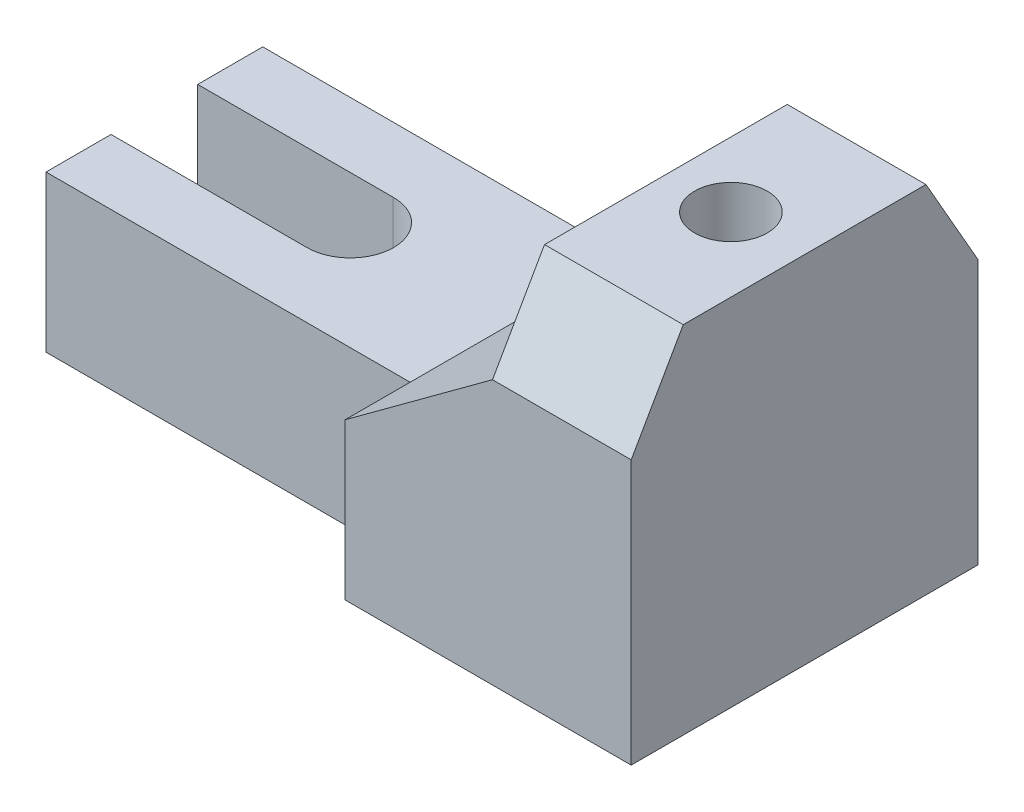
ISO-10303-21;
HEADER;
FILE_DESCRIPTION(('STEP AP214'),'2;1');
FILE_NAME('part.step','',(''),(''),'','','');
FILE_SCHEMA(('AUTOMOTIVE_DESIGN { 1 0 10303 214 1 1 1 1 }'));
ENDSEC;
DATA;
#1=APPLICATION_CONTEXT('core data for automotive mechanical design processes');
#2=APPLICATION_PROTOCOL_DEFINITION('international standard','automotive_design',2000,#1);
#3=PRODUCT_CONTEXT('',#1,'mechanical');
#4=PRODUCT('Part','Part','',(#3));
#5=PRODUCT_RELATED_PRODUCT_CATEGORY('part','',(#4));
#6=PRODUCT_DEFINITION_FORMATION('','',#4);
#7=PRODUCT_DEFINITION_CONTEXT('part definition',#1,'design');
#8=PRODUCT_DEFINITION('design','',#6,#7);
#9=PRODUCT_DEFINITION_SHAPE('','',#8);
#10=(LENGTH_UNIT() NAMED_UNIT(*) SI_UNIT(.MILLI.,.METRE.));
#11=(NAMED_UNIT(*) PLANE_ANGLE_UNIT() SI_UNIT($,.RADIAN.));
#12=(NAMED_UNIT(*) SI_UNIT($,.STERADIAN.) SOLID_ANGLE_UNIT());
#13=UNCERTAINTY_MEASURE_WITH_UNIT(LENGTH_MEASURE(1.E-05),#10,'distance_accuracy_value','');
#14=(GEOMETRIC_REPRESENTATION_CONTEXT(3) GLOBAL_UNCERTAINTY_ASSIGNED_CONTEXT((#13)) GLOBAL_UNIT_ASSIGNED_CONTEXT((#10,
#11,#12)) REPRESENTATION_CONTEXT('',''));
#15=CARTESIAN_POINT('',(0.,0.,0.));
#16=DIRECTION('',(0.,0.,1.));
#17=DIRECTION('',(1.,0.,0.));
#18=AXIS2_PLACEMENT_3D('',#15,#16,#17);
#19=CARTESIAN_POINT('',(-39.,0.,0.));
#20=DIRECTION('',(-1.,0.,0.));
#21=DIRECTION('',(0.,0.,1.));
#22=AXIS2_PLACEMENT_3D('',#19,#20,#21);
#23=PLANE('',#22);
#24=DIRECTION('',(0.,1.,0.));
#25=VECTOR('',#24,1.);
#26=CARTESIAN_POINT('',(-39.,0.,9.99809322082355));
#27=LINE('',#26,#25);
#28=CARTESIAN_POINT('',(-39.,0.,9.99809322082355));
#29=VERTEX_POINT('',#28);
#30=CARTESIAN_POINT('',(-39.,36.,9.99809322082355));
#31=VERTEX_POINT('',#30);
#32=EDGE_CURVE('E11',#29,#31,#27,.T.);
#33=ORIENTED_EDGE('',*,*,#32,.F.);
#34=DIRECTION('',(0.,0.,1.));
#35=VECTOR('',#34,1.);
#36=CARTESIAN_POINT('',(-39.,0.,-10.));
#37=LINE('',#36,#35);
#38=CARTESIAN_POINT('',(-39.,0.,10.));
#39=VERTEX_POINT('',#38);
#40=EDGE_CURVE('E291',#29,#39,#37,.T.);
#41=ORIENTED_EDGE('',*,*,#40,.T.);
#42=DIRECTION('',(0.,1.,0.));
#43=VECTOR('',#42,1.);
#44=CARTESIAN_POINT('',(-39.,36.,9.99999999999999));
#45=LINE('',#44,#43);
#46=CARTESIAN_POINT('',(-39.,36.,9.99999999999999));
#47=VERTEX_POINT('',#46);
#48=EDGE_CURVE('E173',#39,#47,#45,.T.);
#49=ORIENTED_EDGE('',*,*,#48,.T.);
#50=DIRECTION('',(0.,0.,-1.));
#51=VECTOR('',#50,1.);
#52=CARTESIAN_POINT('',(-39.,36.,-10.));
#53=LINE('',#52,#51);
#54=EDGE_CURVE('E170',#47,#31,#53,.T.);
#55=ORIENTED_EDGE('',*,*,#54,.T.);
#56=EDGE_LOOP('',(#33,#41,#49,#55));
#57=FACE_BOUND('',#56,.T.);
#58=ADVANCED_FACE('F39',(#57),#23,.T.);
#59=CARTESIAN_POINT('',(-84.,0.,0.));
#60=DIRECTION('',(-1.,0.,0.));
#61=DIRECTION('',(0.,0.,1.));
#62=AXIS2_PLACEMENT_3D('',#59,#60,#61);
#63=PLANE('',#62);
#64=DIRECTION('',(0.,-1.,0.));
#65=VECTOR('',#64,1.);
#66=CARTESIAN_POINT('',(-84.,36.,-10.));
#67=LINE('',#66,#65);
#68=CARTESIAN_POINT('',(-84.,36.,-10.));
#69=VERTEX_POINT('',#68);
#70=CARTESIAN_POINT('',(-84.,0.,-10.));
#71=VERTEX_POINT('',#70);
#72=EDGE_CURVE('E181',#69,#71,#67,.T.);
#73=ORIENTED_EDGE('',*,*,#72,.F.);
#74=DIRECTION('',(0.,0.,-1.));
#75=VECTOR('',#74,1.);
#76=CARTESIAN_POINT('',(-84.,36.,-25.));
#77=LINE('',#76,#75);
#78=CARTESIAN_POINT('',(-84.,36.,-25.));
#79=VERTEX_POINT('',#78);
#80=EDGE_CURVE('E205',#69,#79,#77,.T.);
#81=ORIENTED_EDGE('',*,*,#80,.T.);
#82=DIRECTION('',(0.,-1.,0.));
#83=VECTOR('',#82,1.);
#84=CARTESIAN_POINT('',(-84.,36.,-25.));
#85=LINE('',#84,#83);
#86=CARTESIAN_POINT('',(-84.,0.,-25.));
#87=VERTEX_POINT('',#86);
#88=EDGE_CURVE('E195',#79,#87,#85,.T.);
#89=ORIENTED_EDGE('',*,*,#88,.T.);
#90=DIRECTION('',(0.,0.,1.));
#91=VECTOR('',#90,1.);
#92=CARTESIAN_POINT('',(-84.,0.,-25.));
#93=LINE('',#92,#91);
#94=EDGE_CURVE('E196',#87,#71,#93,.T.);
#95=ORIENTED_EDGE('',*,*,#94,.T.);
#96=EDGE_LOOP('',(#73,#81,#89,#95));
#97=FACE_BOUND('',#96,.T.);
#98=ADVANCED_FACE('F324',(#97),#63,.T.);
#99=CARTESIAN_POINT('',(0.,0.,40.));
#100=DIRECTION('',(1.,0.,0.));
#101=DIRECTION('',(0.,0.,-1.));
#102=AXIS2_PLACEMENT_3D('',#99,#100,#101);
#103=PLANE('',#102);
#104=DIRECTION('',(0.,-1.,0.));
#105=VECTOR('',#104,1.);
#106=CARTESIAN_POINT('',(0.,36.,-25.));
#107=LINE('',#106,#105);
#108=CARTESIAN_POINT('',(0.,36.,-25.));
#109=VERTEX_POINT('',#108);
#110=CARTESIAN_POINT('',(0.,0.,-25.));
#111=VERTEX_POINT('',#110);
#112=EDGE_CURVE('E189',#109,#111,#107,.T.);
#113=ORIENTED_EDGE('',*,*,#112,.F.);
#114=DIRECTION('',(0.,0.,-1.));
#115=VECTOR('',#114,1.);
#116=CARTESIAN_POINT('',(0.,36.,40.));
#117=LINE('',#116,#115);
#118=CARTESIAN_POINT('',(0.,36.,-40.));
#119=VERTEX_POINT('',#118);
#120=EDGE_CURVE('E278',#109,#119,#117,.T.);
#121=ORIENTED_EDGE('',*,*,#120,.T.);
#122=DIRECTION('',(0.,-1.,0.));
#123=VECTOR('',#122,1.);
#124=CARTESIAN_POINT('',(0.,0.,-40.));
#125=LINE('',#124,#123);
#126=CARTESIAN_POINT('',(0.,0.,-40.));
#127=VERTEX_POINT('',#126);
#128=EDGE_CURVE('E256',#119,#127,#125,.T.);
#129=ORIENTED_EDGE('',*,*,#128,.T.);
#130=DIRECTION('',(0.,0.,-1.));
#131=VECTOR('',#130,1.);
#132=CARTESIAN_POINT('',(0.,0.,40.));
#133=LINE('',#132,#131);
#134=EDGE_CURVE('E266',#111,#127,#133,.T.);
#135=ORIENTED_EDGE('',*,*,#134,.F.);
#136=EDGE_LOOP('',(#113,#121,#129,#135));
#137=FACE_BOUND('',#136,.T.);
#138=ADVANCED_FACE('F327',(#137),#103,.F.);
#139=DIRECTION('',(0.,1.,0.));
#140=VECTOR('',#139,1.);
#141=CARTESIAN_POINT('',(0.,36.,25.));
#142=LINE('',#141,#140);
#143=CARTESIAN_POINT('',(0.,0.,25.));
#144=VERTEX_POINT('',#143);
#145=CARTESIAN_POINT('',(0.,36.,25.));
#146=VERTEX_POINT('',#145);
#147=EDGE_CURVE('E209',#144,#146,#142,.T.);
#148=ORIENTED_EDGE('',*,*,#147,.F.);
#149=CARTESIAN_POINT('',(0.,0.,40.));
#150=VERTEX_POINT('',#149);
#151=EDGE_CURVE('E280',#150,#144,#133,.T.);
#152=ORIENTED_EDGE('',*,*,#151,.F.);
#153=DIRECTION('',(0.,-1.,0.));
#154=VECTOR('',#153,1.);
#155=CARTESIAN_POINT('',(0.,0.,40.));
#156=LINE('',#155,#154);
#157=CARTESIAN_POINT('',(0.,36.,40.));
#158=VERTEX_POINT('',#157);
#159=EDGE_CURVE('E263',#158,#150,#156,.T.);
#160=ORIENTED_EDGE('',*,*,#159,.F.);
#161=EDGE_CURVE('E284',#158,#146,#117,.T.);
#162=ORIENTED_EDGE('',*,*,#161,.T.);
#163=EDGE_LOOP('',(#148,#152,#160,#162));
#164=FACE_BOUND('',#163,.T.);
#165=ADVANCED_FACE('F405',(#164),#103,.F.);
#166=CARTESIAN_POINT('',(66.,0.,40.));
#167=DIRECTION('',(0.,1.,0.));
#168=DIRECTION('',(0.,0.,1.));
#169=AXIS2_PLACEMENT_3D('',#166,#167,#168);
#170=PLANE('',#169);
#171=CARTESIAN_POINT('',(49.,0.,0.));
#172=DIRECTION('',(0.,1.,0.));
#173=DIRECTION('',(0.,0.,1.));
#174=AXIS2_PLACEMENT_3D('',#171,#172,#173);
#175=CIRCLE('',#174,8.38186830152186);
#176=CARTESIAN_POINT('',(49.,0.,-8.38186830152186));
#177=VERTEX_POINT('',#176);
#178=EDGE_CURVE('E167',#177,#177,#175,.T.);
#179=ORIENTED_EDGE('',*,*,#178,.T.);
#180=EDGE_LOOP('',(#179));
#181=FACE_BOUND('',#180,.T.);
#182=ORIENTED_EDGE('',*,*,#40,.F.);
#183=CARTESIAN_POINT('',(-38.8047259676192,0.,0.));
#184=DIRECTION('',(0.,1.,0.));
#185=DIRECTION('',(0.,0.,1.));
#186=AXIS2_PLACEMENT_3D('',#183,#184,#185);
#187=CIRCLE('',#186,10.);
#188=CARTESIAN_POINT('',(-39.,0.,-9.99809322082355));
#189=VERTEX_POINT('',#188);
#190=EDGE_CURVE('E157',#29,#189,#187,.T.);
#191=ORIENTED_EDGE('',*,*,#190,.T.);
#192=CARTESIAN_POINT('',(-39.,0.,-10.));
#193=VERTEX_POINT('',#192);
#194=EDGE_CURVE('E292',#193,#189,#37,.T.);
#195=ORIENTED_EDGE('',*,*,#194,.F.);
#196=DIRECTION('',(-1.,0.,0.));
#197=VECTOR('',#196,1.);
#198=CARTESIAN_POINT('',(-39.,0.,-10.));
#199=LINE('',#198,#197);
#200=EDGE_CURVE('E172',#193,#71,#199,.T.);
#201=ORIENTED_EDGE('',*,*,#200,.T.);
#202=ORIENTED_EDGE('',*,*,#94,.F.);
#203=DIRECTION('',(1.,0.,0.));
#204=VECTOR('',#203,1.);
#205=CARTESIAN_POINT('',(-84.,0.,-25.));
#206=LINE('',#205,#204);
#207=EDGE_CURVE('E225',#87,#111,#206,.T.);
#208=ORIENTED_EDGE('',*,*,#207,.T.);
#209=ORIENTED_EDGE('',*,*,#134,.T.);
#210=DIRECTION('',(1.,0.,0.));
#211=VECTOR('',#210,1.);
#212=CARTESIAN_POINT('',(66.,0.,-40.));
#213=LINE('',#212,#211);
#214=CARTESIAN_POINT('',(66.,0.,-40.));
#215=VERTEX_POINT('',#214);
#216=EDGE_CURVE('E251',#127,#215,#213,.T.);
#217=ORIENTED_EDGE('',*,*,#216,.T.);
#218=DIRECTION('',(0.,0.,-1.));
#219=VECTOR('',#218,1.);
#220=CARTESIAN_POINT('',(66.,0.,40.));
#221=LINE('',#220,#219);
#222=CARTESIAN_POINT('',(66.,0.,40.));
#223=VERTEX_POINT('',#222);
#224=EDGE_CURVE('E286',#223,#215,#221,.T.);
#225=ORIENTED_EDGE('',*,*,#224,.F.);
#226=DIRECTION('',(1.,0.,0.));
#227=VECTOR('',#226,1.);
#228=CARTESIAN_POINT('',(66.,0.,40.));
#229=LINE('',#228,#227);
#230=EDGE_CURVE('E253',#150,#223,#229,.T.);
#231=ORIENTED_EDGE('',*,*,#230,.F.);
#232=ORIENTED_EDGE('',*,*,#151,.T.);
#233=DIRECTION('',(1.,0.,0.));
#234=VECTOR('',#233,1.);
#235=CARTESIAN_POINT('',(-84.,0.,25.));
#236=LINE('',#235,#234);
#237=CARTESIAN_POINT('',(-84.,0.,25.));
#238=VERTEX_POINT('',#237);
#239=EDGE_CURVE('E218',#238,#144,#236,.T.);
#240=ORIENTED_EDGE('',*,*,#239,.F.);
#241=CARTESIAN_POINT('',(-84.,0.,10.));
#242=VERTEX_POINT('',#241);
#243=EDGE_CURVE('E193',#242,#238,#93,.T.);
#244=ORIENTED_EDGE('',*,*,#243,.F.);
#245=DIRECTION('',(-1.,0.,0.));
#246=VECTOR('',#245,1.);
#247=CARTESIAN_POINT('',(-39.,0.,10.));
#248=LINE('',#247,#246);
#249=EDGE_CURVE('E62',#39,#242,#248,.T.);
#250=ORIENTED_EDGE('',*,*,#249,.F.);
#251=EDGE_LOOP('',(#182,#191,#195,#201,#202,#208,#209,#217,#225,#231,#232,#240,#244,#250));
#252=FACE_BOUND('',#251,.T.);
#253=ADVANCED_FACE('F41',(#181,#252),#170,.F.);
#254=CARTESIAN_POINT('',(66.,61.,40.));
#255=DIRECTION('',(-1.,0.,0.));
#256=DIRECTION('',(0.,-1.,0.));
#257=AXIS2_PLACEMENT_3D('',#254,#255,#256);
#258=PLANE('',#257);
#259=DIRECTION('',(0.,0.,-1.));
#260=VECTOR('',#259,1.);
#261=CARTESIAN_POINT('',(66.,82.,-40.));
#262=LINE('',#261,#260);
#263=CARTESIAN_POINT('',(66.,82.,28.));
#264=VERTEX_POINT('',#263);
#265=CARTESIAN_POINT('',(66.,82.,-28.));
#266=VERTEX_POINT('',#265);
#267=EDGE_CURVE('E252',#264,#266,#262,.T.);
#268=ORIENTED_EDGE('',*,*,#267,.F.);
#269=DIRECTION('',(0.,0.868243142124459,-0.496138938356834));
#270=VECTOR('',#269,1.);
#271=CARTESIAN_POINT('',(66.,61.,40.));
#272=LINE('',#271,#270);
#273=CARTESIAN_POINT('',(66.,61.,40.));
#274=VERTEX_POINT('',#273);
#275=EDGE_CURVE('E229',#274,#264,#272,.T.);
#276=ORIENTED_EDGE('',*,*,#275,.F.);
#277=DIRECTION('',(0.,1.,0.));
#278=VECTOR('',#277,1.);
#279=CARTESIAN_POINT('',(66.,61.,40.));
#280=LINE('',#279,#278);
#281=EDGE_CURVE('E259',#223,#274,#280,.T.);
#282=ORIENTED_EDGE('',*,*,#281,.F.);
#283=ORIENTED_EDGE('',*,*,#224,.T.);
#284=DIRECTION('',(0.,1.,0.));
#285=VECTOR('',#284,1.);
#286=CARTESIAN_POINT('',(66.,61.,-40.));
#287=LINE('',#286,#285);
#288=CARTESIAN_POINT('',(66.,61.,-40.));
#289=VERTEX_POINT('',#288);
#290=EDGE_CURVE('E268',#215,#289,#287,.T.);
#291=ORIENTED_EDGE('',*,*,#290,.T.);
#292=DIRECTION('',(0.,-0.868243142124459,-0.496138938356834));
#293=VECTOR('',#292,1.);
#294=CARTESIAN_POINT('',(66.,61.,-40.));
#295=LINE('',#294,#293);
#296=EDGE_CURVE('E235',#266,#289,#295,.T.);
#297=ORIENTED_EDGE('',*,*,#296,.F.);
#298=EDGE_LOOP('',(#268,#276,#282,#283,#291,#297));
#299=FACE_BOUND('',#298,.T.);
#300=ADVANCED_FACE('F373',(#299),#258,.F.);
#301=CARTESIAN_POINT('',(0.,36.,40.));
#302=DIRECTION('',(0.592390450477518,-0.805651012649425,0.));
#303=DIRECTION('',(0.805651012649425,0.592390450477518,0.));
#304=AXIS2_PLACEMENT_3D('',#301,#302,#303);
#305=PLANE('',#304);
#306=DIRECTION('',(-0.805651012649425,-0.592390450477518,0.));
#307=VECTOR('',#306,1.);
#308=CARTESIAN_POINT('',(0.,36.,-40.));
#309=LINE('',#308,#307);
#310=CARTESIAN_POINT('',(34.,61.,-40.));
#311=VERTEX_POINT('',#310);
#312=EDGE_CURVE('E275',#311,#119,#309,.T.);
#313=ORIENTED_EDGE('',*,*,#312,.T.);
#314=ORIENTED_EDGE('',*,*,#120,.F.);
#315=DIRECTION('',(0.,0.,-1.));
#316=VECTOR('',#315,1.);
#317=CARTESIAN_POINT('',(0.,36.,-25.));
#318=LINE('',#317,#316);
#319=EDGE_CURVE('E199',#146,#109,#318,.T.);
#320=ORIENTED_EDGE('',*,*,#319,.F.);
#321=ORIENTED_EDGE('',*,*,#161,.F.);
#322=DIRECTION('',(-0.805651012649425,-0.592390450477518,0.));
#323=VECTOR('',#322,1.);
#324=CARTESIAN_POINT('',(0.,36.,40.));
#325=LINE('',#324,#323);
#326=CARTESIAN_POINT('',(34.,61.,40.));
#327=VERTEX_POINT('',#326);
#328=EDGE_CURVE('E261',#327,#158,#325,.T.);
#329=ORIENTED_EDGE('',*,*,#328,.F.);
#330=DIRECTION('',(0.,0.,-1.));
#331=VECTOR('',#330,1.);
#332=CARTESIAN_POINT('',(34.,61.,40.));
#333=LINE('',#332,#331);
#334=EDGE_CURVE('E285',#327,#311,#333,.T.);
#335=ORIENTED_EDGE('',*,*,#334,.T.);
#336=EDGE_LOOP('',(#313,#314,#320,#321,#329,#335));
#337=FACE_BOUND('',#336,.T.);
#338=ADVANCED_FACE('F384',(#337),#305,.F.);
#339=CARTESIAN_POINT('',(0.,0.,40.));
#340=DIRECTION('',(0.,0.,-1.));
#341=DIRECTION('',(-1.,0.,0.));
#342=AXIS2_PLACEMENT_3D('',#339,#340,#341);
#343=PLANE('',#342);
#344=ORIENTED_EDGE('',*,*,#281,.T.);
#345=DIRECTION('',(1.,0.,0.));
#346=VECTOR('',#345,1.);
#347=CARTESIAN_POINT('',(34.,61.,40.));
#348=LINE('',#347,#346);
#349=EDGE_CURVE('E230',#327,#274,#348,.T.);
#350=ORIENTED_EDGE('',*,*,#349,.F.);
#351=ORIENTED_EDGE('',*,*,#328,.T.);
#352=ORIENTED_EDGE('',*,*,#159,.T.);
#353=ORIENTED_EDGE('',*,*,#230,.T.);
#354=EDGE_LOOP('',(#344,#350,#351,#352,#353));
#355=FACE_BOUND('',#354,.T.);
#356=ADVANCED_FACE('F387',(#355),#343,.F.);
#357=CARTESIAN_POINT('',(0.,0.,-40.));
#358=DIRECTION('',(0.,0.,-1.));
#359=DIRECTION('',(-1.,0.,0.));
#360=AXIS2_PLACEMENT_3D('',#357,#358,#359);
#361=PLANE('',#360);
#362=DIRECTION('',(1.,0.,0.));
#363=VECTOR('',#362,1.);
#364=CARTESIAN_POINT('',(34.,61.,-40.));
#365=LINE('',#364,#363);
#366=EDGE_CURVE('E224',#311,#289,#365,.T.);
#367=ORIENTED_EDGE('',*,*,#366,.T.);
#368=ORIENTED_EDGE('',*,*,#290,.F.);
#369=ORIENTED_EDGE('',*,*,#216,.F.);
#370=ORIENTED_EDGE('',*,*,#128,.F.);
#371=ORIENTED_EDGE('',*,*,#312,.F.);
#372=EDGE_LOOP('',(#367,#368,#369,#370,#371));
#373=FACE_BOUND('',#372,.T.);
#374=ADVANCED_FACE('F376',(#373),#361,.T.);
#375=CARTESIAN_POINT('',(0.,82.,0.));
#376=DIRECTION('',(0.,-1.,0.));
#377=DIRECTION('',(0.,0.,-1.));
#378=AXIS2_PLACEMENT_3D('',#375,#376,#377);
#379=PLANE('',#378);
#380=DIRECTION('',(0.,0.,1.));
#381=VECTOR('',#380,1.);
#382=CARTESIAN_POINT('',(34.,82.,40.));
#383=LINE('',#382,#381);
#384=CARTESIAN_POINT('',(34.,82.,-28.));
#385=VERTEX_POINT('',#384);
#386=CARTESIAN_POINT('',(34.,82.,28.));
#387=VERTEX_POINT('',#386);
#388=EDGE_CURVE('E247',#385,#387,#383,.T.);
#389=ORIENTED_EDGE('',*,*,#388,.T.);
#390=DIRECTION('',(1.,0.,0.));
#391=VECTOR('',#390,1.);
#392=CARTESIAN_POINT('',(34.,82.,28.));
#393=LINE('',#392,#391);
#394=EDGE_CURVE('E231',#387,#264,#393,.T.);
#395=ORIENTED_EDGE('',*,*,#394,.T.);
#396=ORIENTED_EDGE('',*,*,#267,.T.);
#397=DIRECTION('',(1.,0.,0.));
#398=VECTOR('',#397,1.);
#399=CARTESIAN_POINT('',(34.,82.,-28.));
#400=LINE('',#399,#398);
#401=EDGE_CURVE('E238',#385,#266,#400,.T.);
#402=ORIENTED_EDGE('',*,*,#401,.F.);
#403=EDGE_LOOP('',(#389,#395,#396,#402));
#404=FACE_BOUND('',#403,.T.);
#405=CARTESIAN_POINT('',(49.,82.,0.));
#406=DIRECTION('',(0.,1.,0.));
#407=DIRECTION('',(0.,0.,1.));
#408=AXIS2_PLACEMENT_3D('',#405,#406,#407);
#409=CIRCLE('',#408,8.38186830152186);
#410=CARTESIAN_POINT('',(49.,82.,-8.38186830152186));
#411=VERTEX_POINT('',#410);
#412=EDGE_CURVE('E236',#411,#411,#409,.T.);
#413=ORIENTED_EDGE('',*,*,#412,.F.);
#414=EDGE_LOOP('',(#413));
#415=FACE_BOUND('',#414,.T.);
#416=ADVANCED_FACE('F319',(#404,#415),#379,.F.);
#417=CARTESIAN_POINT('',(34.,82.,40.));
#418=DIRECTION('',(1.,0.,0.));
#419=DIRECTION('',(0.,0.,-1.));
#420=AXIS2_PLACEMENT_3D('',#417,#418,#419);
#421=PLANE('',#420);
#422=ORIENTED_EDGE('',*,*,#334,.F.);
#423=DIRECTION('',(0.,0.868243142124459,-0.496138938356834));
#424=VECTOR('',#423,1.);
#425=CARTESIAN_POINT('',(34.,61.,40.));
#426=LINE('',#425,#424);
#427=EDGE_CURVE('E228',#327,#387,#426,.T.);
#428=ORIENTED_EDGE('',*,*,#427,.T.);
#429=ORIENTED_EDGE('',*,*,#388,.F.);
#430=DIRECTION('',(0.,-0.868243142124459,-0.496138938356834));
#431=VECTOR('',#430,1.);
#432=CARTESIAN_POINT('',(34.,61.,-40.));
#433=LINE('',#432,#431);
#434=EDGE_CURVE('E239',#385,#311,#433,.T.);
#435=ORIENTED_EDGE('',*,*,#434,.T.);
#436=EDGE_LOOP('',(#422,#428,#429,#435));
#437=FACE_BOUND('',#436,.T.);
#438=ADVANCED_FACE('F310',(#437),#421,.F.);
#439=CARTESIAN_POINT('',(49.,82.,0.));
#440=DIRECTION('',(0.,-1.,0.));
#441=DIRECTION('',(0.,0.,-1.));
#442=AXIS2_PLACEMENT_3D('',#439,#440,#441);
#443=CYLINDRICAL_SURFACE('',#442,8.38186830152186);
#444=CARTESIAN_POINT('',(49.,82.,-8.38186830152186));
#445=CARTESIAN_POINT('',(49.,81.1458333333333,-8.38186830152186));
#446=CARTESIAN_POINT('',(49.,80.2916666666667,-8.38186830152186));
#447=CARTESIAN_POINT('',(49.,78.5833333333333,-8.38186830152186));
#448=CARTESIAN_POINT('',(49.,77.7291666666667,-8.38186830152186));
#449=CARTESIAN_POINT('',(49.,76.0208333333333,-8.38186830152186));
#450=CARTESIAN_POINT('',(49.,75.1666666666667,-8.38186830152186));
#451=CARTESIAN_POINT('',(49.,73.4583333333333,-8.38186830152186));
#452=CARTESIAN_POINT('',(49.,72.6041666666667,-8.38186830152186));
#453=CARTESIAN_POINT('',(49.,70.8958333333333,-8.38186830152186));
#454=CARTESIAN_POINT('',(49.,70.0416666666667,-8.38186830152186));
#455=CARTESIAN_POINT('',(49.,68.3333333333333,-8.38186830152186));
#456=CARTESIAN_POINT('',(49.,67.4791666666667,-8.38186830152186));
#457=CARTESIAN_POINT('',(49.,65.7708333333333,-8.38186830152186));
#458=CARTESIAN_POINT('',(49.,64.9166666666667,-8.38186830152186));
#459=CARTESIAN_POINT('',(49.,63.2083333333333,-8.38186830152186));
#460=CARTESIAN_POINT('',(49.,62.3541666666667,-8.38186830152186));
#461=CARTESIAN_POINT('',(49.,60.6458333333333,-8.38186830152186));
#462=CARTESIAN_POINT('',(49.,59.7916666666667,-8.38186830152186));
#463=CARTESIAN_POINT('',(49.,58.0833333333333,-8.38186830152186));
#464=CARTESIAN_POINT('',(49.,57.2291666666667,-8.38186830152186));
#465=CARTESIAN_POINT('',(49.,55.5208333333333,-8.38186830152186));
#466=CARTESIAN_POINT('',(49.,54.6666666666667,-8.38186830152186));
#467=CARTESIAN_POINT('',(49.,52.9583333333333,-8.38186830152186));
#468=CARTESIAN_POINT('',(49.,52.1041666666667,-8.38186830152186));
#469=CARTESIAN_POINT('',(49.,50.3958333333333,-8.38186830152186));
#470=CARTESIAN_POINT('',(49.,49.5416666666667,-8.38186830152186));
#471=CARTESIAN_POINT('',(49.,47.8333333333333,-8.38186830152186));
#472=CARTESIAN_POINT('',(49.,46.9791666666667,-8.38186830152186));
#473=CARTESIAN_POINT('',(49.,45.2708333333333,-8.38186830152186));
#474=CARTESIAN_POINT('',(49.,44.4166666666667,-8.38186830152186));
#475=CARTESIAN_POINT('',(49.,42.7083333333333,-8.38186830152186));
#476=CARTESIAN_POINT('',(49.,41.8541666666667,-8.38186830152186));
#477=CARTESIAN_POINT('',(49.,40.1458333333333,-8.38186830152186));
#478=CARTESIAN_POINT('',(49.,39.2916666666667,-8.38186830152186));
#479=CARTESIAN_POINT('',(49.,37.5833333333333,-8.38186830152186));
#480=CARTESIAN_POINT('',(49.,36.7291666666667,-8.38186830152186));
#481=CARTESIAN_POINT('',(49.,35.0208333333333,-8.38186830152186));
#482=CARTESIAN_POINT('',(49.,34.1666666666667,-8.38186830152186));
#483=CARTESIAN_POINT('',(49.,32.4583333333333,-8.38186830152186));
#484=CARTESIAN_POINT('',(49.,31.6041666666667,-8.38186830152186));
#485=CARTESIAN_POINT('',(49.,29.8958333333333,-8.38186830152186));
#486=CARTESIAN_POINT('',(49.,29.0416666666667,-8.38186830152186));
#487=CARTESIAN_POINT('',(49.,27.3333333333333,-8.38186830152186));
#488=CARTESIAN_POINT('',(49.,26.4791666666667,-8.38186830152186));
#489=CARTESIAN_POINT('',(49.,24.7708333333333,-8.38186830152186));
#490=CARTESIAN_POINT('',(49.,23.9166666666667,-8.38186830152186));
#491=CARTESIAN_POINT('',(49.,22.2083333333333,-8.38186830152186));
#492=CARTESIAN_POINT('',(49.,21.3541666666667,-8.38186830152186));
#493=CARTESIAN_POINT('',(49.,19.6458333333333,-8.38186830152186));
#494=CARTESIAN_POINT('',(49.,18.7916666666667,-8.38186830152186));
#495=CARTESIAN_POINT('',(49.,17.0833333333333,-8.38186830152186));
#496=CARTESIAN_POINT('',(49.,16.2291666666667,-8.38186830152186));
#497=CARTESIAN_POINT('',(49.,14.5208333333333,-8.38186830152186));
#498=CARTESIAN_POINT('',(49.,13.6666666666667,-8.38186830152186));
#499=CARTESIAN_POINT('',(49.,11.9583333333333,-8.38186830152186));
#500=CARTESIAN_POINT('',(49.,11.1041666666667,-8.38186830152186));
#501=CARTESIAN_POINT('',(49.,9.39583333333334,-8.38186830152186));
#502=CARTESIAN_POINT('',(49.,8.54166666666667,-8.38186830152186));
#503=CARTESIAN_POINT('',(49.,6.83333333333333,-8.38186830152186));
#504=CARTESIAN_POINT('',(49.,5.97916666666667,-8.38186830152186));
#505=CARTESIAN_POINT('',(49.,4.27083333333333,-8.38186830152186));
#506=CARTESIAN_POINT('',(49.,3.41666666666667,-8.38186830152186));
#507=CARTESIAN_POINT('',(49.,1.70833333333333,-8.38186830152186));
#508=CARTESIAN_POINT('',(49.,0.854166666666665,-8.38186830152186));
#509=CARTESIAN_POINT('',(49.,0.,-8.38186830152186));
#510=B_SPLINE_CURVE_WITH_KNOTS('',3,(#444,#445,#446,#447,#448,#449,#450,#451,#452,#453,#454,
#455,#456,#457,#458,#459,#460,#461,#462,#463,#464,#465,#466,#467,#468,#469,#470,#471,#472,#473,
#474,#475,#476,#477,#478,#479,#480,#481,#482,#483,#484,#485,#486,#487,#488,#489,#490,#491,#492,
#493,#494,#495,#496,#497,#498,#499,#500,#501,#502,#503,#504,#505,#506,#507,#508,#509),
.UNSPECIFIED.,.F.,.F.,(4,2,2,2,2,2,2,2,2,2,2,2,2,2,2,2,2,2,2,2,2,2,2,2,2,2,2,2,2,2,2,2,4),(0.,
2.56250000000001,5.125,7.68750000000001,10.25,12.8125,15.375,17.9375,20.5,23.0625,25.625,
28.1875,30.75,33.3125,35.875,38.4375,41.,43.5625,46.125,48.6875,51.25,53.8125,56.375,58.9375,
61.5,64.0625,66.625,69.1875,71.75,74.3125,76.875,79.4375,82.),.UNSPECIFIED.);
#511=EDGE_CURVE('BSEAM302',#411,#177,#510,.T.);
#512=ORIENTED_EDGE('',*,*,#412,.T.);
#513=ORIENTED_EDGE('',*,*,#178,.F.);
#514=ORIENTED_EDGE('',*,*,#511,.T.);
#515=ORIENTED_EDGE('',*,*,#511,.F.);
#516=EDGE_LOOP('',(#512,#514,#513,#515));
#517=FACE_BOUND('',#516,.T.);
#518=ADVANCED_FACE('F302',(#517),#443,.F.);
#519=CARTESIAN_POINT('',(34.,61.,-40.));
#520=DIRECTION('',(0.,-0.496138938356834,0.868243142124459));
#521=DIRECTION('',(0.,-0.868243142124459,-0.496138938356834));
#522=AXIS2_PLACEMENT_3D('',#519,#520,#521);
#523=PLANE('',#522);
#524=ORIENTED_EDGE('',*,*,#296,.T.);
#525=ORIENTED_EDGE('',*,*,#366,.F.);
#526=ORIENTED_EDGE('',*,*,#434,.F.);
#527=ORIENTED_EDGE('',*,*,#401,.T.);
#528=EDGE_LOOP('',(#524,#525,#526,#527));
#529=FACE_BOUND('',#528,.T.);
#530=ADVANCED_FACE('F306',(#529),#523,.F.);
#531=CARTESIAN_POINT('',(34.,61.,40.));
#532=DIRECTION('',(0.,-0.496138938356834,-0.868243142124459));
#533=DIRECTION('',(0.,0.868243142124459,-0.496138938356834));
#534=AXIS2_PLACEMENT_3D('',#531,#532,#533);
#535=PLANE('',#534);
#536=ORIENTED_EDGE('',*,*,#275,.T.);
#537=ORIENTED_EDGE('',*,*,#394,.F.);
#538=ORIENTED_EDGE('',*,*,#427,.F.);
#539=ORIENTED_EDGE('',*,*,#349,.T.);
#540=EDGE_LOOP('',(#536,#537,#538,#539));
#541=FACE_BOUND('',#540,.T.);
#542=ADVANCED_FACE('F313',(#541),#535,.F.);
#543=CARTESIAN_POINT('',(-84.,36.,-25.));
#544=DIRECTION('',(0.,0.,1.));
#545=DIRECTION('',(1.,0.,0.));
#546=AXIS2_PLACEMENT_3D('',#543,#544,#545);
#547=PLANE('',#546);
#548=ORIENTED_EDGE('',*,*,#112,.T.);
#549=ORIENTED_EDGE('',*,*,#207,.F.);
#550=ORIENTED_EDGE('',*,*,#88,.F.);
#551=DIRECTION('',(1.,0.,0.));
#552=VECTOR('',#551,1.);
#553=CARTESIAN_POINT('',(-84.,36.,-25.));
#554=LINE('',#553,#552);
#555=EDGE_CURVE('E207',#79,#109,#554,.T.);
#556=ORIENTED_EDGE('',*,*,#555,.T.);
#557=EDGE_LOOP('',(#548,#549,#550,#556));
#558=FACE_BOUND('',#557,.T.);
#559=ADVANCED_FACE('F353',(#558),#547,.F.);
#560=CARTESIAN_POINT('',(-84.,36.,25.));
#561=DIRECTION('',(0.,0.,-1.));
#562=DIRECTION('',(0.,1.,0.));
#563=AXIS2_PLACEMENT_3D('',#560,#561,#562);
#564=PLANE('',#563);
#565=ORIENTED_EDGE('',*,*,#147,.T.);
#566=DIRECTION('',(1.,0.,0.));
#567=VECTOR('',#566,1.);
#568=CARTESIAN_POINT('',(-84.,36.,25.));
#569=LINE('',#568,#567);
#570=CARTESIAN_POINT('',(-84.,36.,25.));
#571=VERTEX_POINT('',#570);
#572=EDGE_CURVE('E219',#571,#146,#569,.T.);
#573=ORIENTED_EDGE('',*,*,#572,.F.);
#574=DIRECTION('',(0.,1.,0.));
#575=VECTOR('',#574,1.);
#576=CARTESIAN_POINT('',(-84.,36.,25.));
#577=LINE('',#576,#575);
#578=EDGE_CURVE('E197',#238,#571,#577,.T.);
#579=ORIENTED_EDGE('',*,*,#578,.F.);
#580=ORIENTED_EDGE('',*,*,#239,.T.);
#581=EDGE_LOOP('',(#565,#573,#579,#580));
#582=FACE_BOUND('',#581,.T.);
#583=ADVANCED_FACE('F351',(#582),#564,.F.);
#584=CARTESIAN_POINT('',(-84.,36.,-25.));
#585=DIRECTION('',(0.,-1.,0.));
#586=DIRECTION('',(0.,0.,-1.));
#587=AXIS2_PLACEMENT_3D('',#584,#585,#586);
#588=PLANE('',#587);
#589=CARTESIAN_POINT('',(-39.,36.,-9.99809322082355));
#590=VERTEX_POINT('',#589);
#591=CARTESIAN_POINT('',(-39.,36.,-10.));
#592=VERTEX_POINT('',#591);
#593=EDGE_CURVE('E169',#590,#592,#53,.T.);
#594=ORIENTED_EDGE('',*,*,#593,.F.);
#595=CARTESIAN_POINT('',(-38.8047259676192,36.,0.));
#596=DIRECTION('',(0.,1.,0.));
#597=DIRECTION('',(0.,0.,1.));
#598=AXIS2_PLACEMENT_3D('',#595,#596,#597);
#599=CIRCLE('',#598,10.);
#600=EDGE_CURVE('E52',#31,#590,#599,.T.);
#601=ORIENTED_EDGE('',*,*,#600,.F.);
#602=ORIENTED_EDGE('',*,*,#54,.F.);
#603=DIRECTION('',(-1.,0.,0.));
#604=VECTOR('',#603,1.);
#605=CARTESIAN_POINT('',(-39.,36.,9.99999999999999));
#606=LINE('',#605,#604);
#607=CARTESIAN_POINT('',(-84.,36.,9.99999999999999));
#608=VERTEX_POINT('',#607);
#609=EDGE_CURVE('E186',#47,#608,#606,.T.);
#610=ORIENTED_EDGE('',*,*,#609,.T.);
#611=EDGE_CURVE('E202',#571,#608,#77,.T.);
#612=ORIENTED_EDGE('',*,*,#611,.F.);
#613=ORIENTED_EDGE('',*,*,#572,.T.);
#614=ORIENTED_EDGE('',*,*,#319,.T.);
#615=ORIENTED_EDGE('',*,*,#555,.F.);
#616=ORIENTED_EDGE('',*,*,#80,.F.);
#617=DIRECTION('',(-1.,0.,0.));
#618=VECTOR('',#617,1.);
#619=CARTESIAN_POINT('',(-39.,36.,-10.));
#620=LINE('',#619,#618);
#621=EDGE_CURVE('E187',#592,#69,#620,.T.);
#622=ORIENTED_EDGE('',*,*,#621,.F.);
#623=EDGE_LOOP('',(#594,#601,#602,#610,#612,#613,#614,#615,#616,#622));
#624=FACE_BOUND('',#623,.T.);
#625=ADVANCED_FACE('F164',(#624),#588,.F.);
#626=DIRECTION('',(0.,1.,0.));
#627=VECTOR('',#626,1.);
#628=CARTESIAN_POINT('',(-84.,36.,9.99999999999999));
#629=LINE('',#628,#627);
#630=EDGE_CURVE('E182',#242,#608,#629,.T.);
#631=ORIENTED_EDGE('',*,*,#630,.F.);
#632=ORIENTED_EDGE('',*,*,#243,.T.);
#633=ORIENTED_EDGE('',*,*,#578,.T.);
#634=ORIENTED_EDGE('',*,*,#611,.T.);
#635=EDGE_LOOP('',(#631,#632,#633,#634));
#636=FACE_BOUND('',#635,.T.);
#637=ADVANCED_FACE('F332',(#636),#63,.T.);
#638=CARTESIAN_POINT('',(-39.,36.,-10.));
#639=DIRECTION('',(0.,0.,-1.));
#640=DIRECTION('',(0.,1.,0.));
#641=AXIS2_PLACEMENT_3D('',#638,#639,#640);
#642=PLANE('',#641);
#643=ORIENTED_EDGE('',*,*,#72,.T.);
#644=ORIENTED_EDGE('',*,*,#200,.F.);
#645=DIRECTION('',(0.,-1.,0.));
#646=VECTOR('',#645,1.);
#647=CARTESIAN_POINT('',(-39.,36.,-10.));
#648=LINE('',#647,#646);
#649=EDGE_CURVE('E184',#592,#193,#648,.T.);
#650=ORIENTED_EDGE('',*,*,#649,.F.);
#651=ORIENTED_EDGE('',*,*,#621,.T.);
#652=EDGE_LOOP('',(#643,#644,#650,#651));
#653=FACE_BOUND('',#652,.T.);
#654=ADVANCED_FACE('F342',(#653),#642,.F.);
#655=CARTESIAN_POINT('',(-39.,36.,9.99999999999999));
#656=DIRECTION('',(0.,0.,1.));
#657=DIRECTION('',(0.,-1.,0.));
#658=AXIS2_PLACEMENT_3D('',#655,#656,#657);
#659=PLANE('',#658);
#660=ORIENTED_EDGE('',*,*,#630,.T.);
#661=ORIENTED_EDGE('',*,*,#609,.F.);
#662=ORIENTED_EDGE('',*,*,#48,.F.);
#663=ORIENTED_EDGE('',*,*,#249,.T.);
#664=EDGE_LOOP('',(#660,#661,#662,#663));
#665=FACE_BOUND('',#664,.T.);
#666=ADVANCED_FACE('F340',(#665),#659,.F.);
#667=DIRECTION('',(0.,1.,0.));
#668=VECTOR('',#667,1.);
#669=CARTESIAN_POINT('',(-39.,0.,-9.99809322082355));
#670=LINE('',#669,#668);
#671=EDGE_CURVE('E50',#590,#189,#670,.F.);
#672=ORIENTED_EDGE('',*,*,#671,.F.);
#673=ORIENTED_EDGE('',*,*,#593,.T.);
#674=ORIENTED_EDGE('',*,*,#649,.T.);
#675=ORIENTED_EDGE('',*,*,#194,.T.);
#676=EDGE_LOOP('',(#672,#673,#674,#675));
#677=FACE_BOUND('',#676,.T.);
#678=ADVANCED_FACE('F298',(#677),#23,.T.);
#679=CARTESIAN_POINT('',(-38.8047259676192,0.,0.));
#680=DIRECTION('',(0.,1.,0.));
#681=DIRECTION('',(0.,0.,1.));
#682=AXIS2_PLACEMENT_3D('',#679,#680,#681);
#683=CYLINDRICAL_SURFACE('',#682,10.);
#684=ORIENTED_EDGE('',*,*,#32,.T.);
#685=ORIENTED_EDGE('',*,*,#600,.T.);
#686=ORIENTED_EDGE('',*,*,#671,.T.);
#687=ORIENTED_EDGE('',*,*,#190,.F.);
#688=EDGE_LOOP('',(#684,#685,#686,#687));
#689=FACE_BOUND('',#688,.T.);
#690=ADVANCED_FACE('F156',(#689),#683,.F.);
#691=CLOSED_SHELL('',(#58,#98,#138,#165,#253,#300,#338,#356,#374,#416,#438,#518,#530,#542,#559,
#583,#625,#637,#654,#666,#678,#690));
#692=MANIFOLD_SOLID_BREP('B2',#691);
#693=ADVANCED_BREP_SHAPE_REPRESENTATION('',(#18,#692),#14);
#694=SHAPE_DEFINITION_REPRESENTATION(#9,#693);
ENDSEC;
END-ISO-10303-21;
